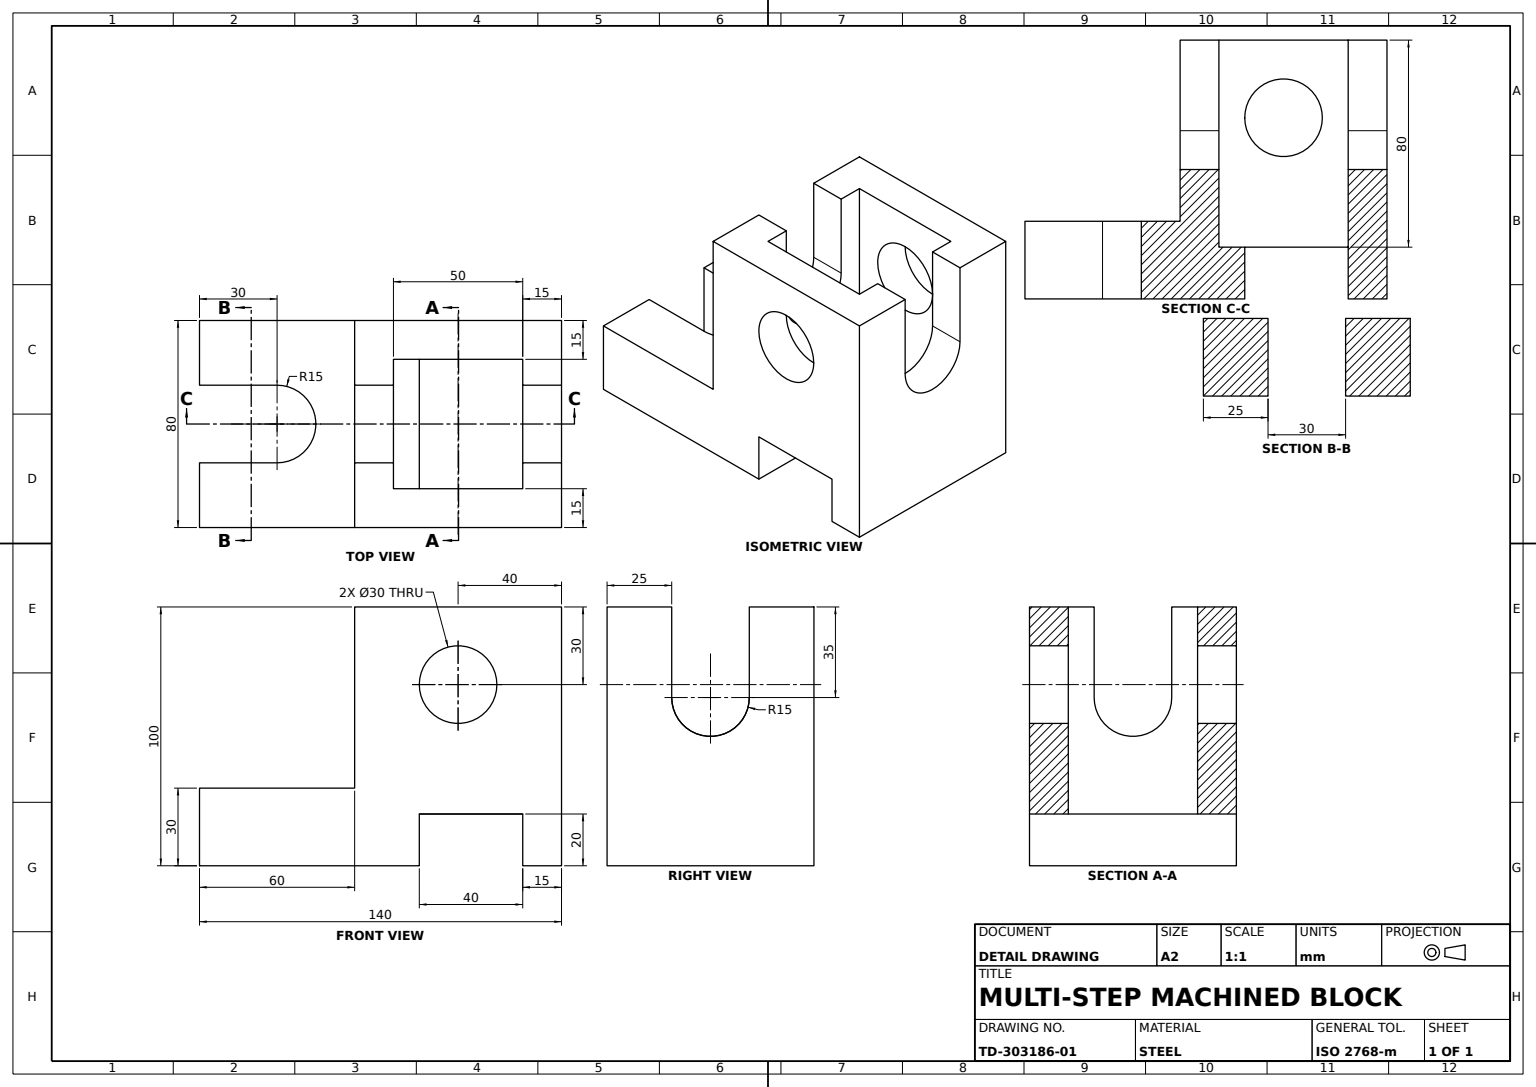
from build123d import *

# Parameters (mm, degrees)
BASE_BLOCK_SKETCH_W             = 140
BASE_BLOCK_SKETCH_H             = 30
BASE_BLOCK_DEPTH                = 80
BASE_NOTCH_SKETCH_W             = 40
BASE_NOTCH_SKETCH_H             = 20
BASE_NOTCH_DEPTH                = 80
UPRIGHT_SKETCH_W                = 80
UPRIGHT_SKETCH_H                = 70
UPRIGHT_DEPTH                   = 80
UPRIGHT_PROFILE_CUT_DEPTH       = 80
CROSS_HOLE_SKETCH_R             = 15
CROSS_HOLE_DEPTH                = 80
UPRIGHT_U_SLOT_DEPTH            = 80
BASE_UNDERSIDE_NOTCH_DEPTH      = 10
BASE_UNDERSIDE_NOTCH_DEPTH_BACK = 80


with BuildPart() as part:
    # Base Block Sketch → Base Block (new body)
    with BuildSketch(Plane.XY):
        with Locations((70, 15)):
            Rectangle(BASE_BLOCK_SKETCH_W, BASE_BLOCK_SKETCH_H)
    extrude(amount=-BASE_BLOCK_DEPTH)

    # Base Notch Sketch → Base Notch (cut)
    with BuildSketch(Plane.XY):
        with Locations((105, 10)):
            Rectangle(BASE_NOTCH_SKETCH_W, BASE_NOTCH_SKETCH_H)
    extrude(amount=-BASE_NOTCH_DEPTH, mode=Mode.SUBTRACT)

    # Upright Sketch → Upright (add)
    with BuildSketch(Plane.XY):
        with Locations((100, 65)):
            Rectangle(UPRIGHT_SKETCH_W, UPRIGHT_SKETCH_H)
    extrude(amount=-UPRIGHT_DEPTH)

    # Upright Profile Cut Sketch → Upright Profile Cut (cut)
    with BuildSketch(Plane(origin=(0, 100, 0), x_dir=(1, 0, 0), z_dir=(0, 1, 0))):
        Polygon((75, 15), (75, 40), (75, 65), (125, 65), (125, 15), align=None)
    extrude(amount=-UPRIGHT_PROFILE_CUT_DEPTH, mode=Mode.SUBTRACT)

    # Cross Hole Sketch → Cross Hole (cut)
    with BuildSketch(Plane.XY):
        with Locations((100, 70)):
            Circle(CROSS_HOLE_SKETCH_R)
    extrude(amount=-CROSS_HOLE_DEPTH, mode=Mode.SUBTRACT)

    # Upright U-Slot Sketch → Upright U-Slot (cut)
    with BuildSketch(Plane.ZY.offset(-60)):
        with BuildLine():
            Line((-25, 100), (-55, 100))
            Line((-55, 100), (-55, 65))
            ThreePointArc((-55, 65), (-40, 50), (-25, 65))
            Line((-25, 65), (-25, 100))
        make_face()
    extrude(amount=-UPRIGHT_U_SLOT_DEPTH, mode=Mode.SUBTRACT)

    # Base Underside Notch Sketch → Base Underside Notch (cut, two sides: drawn at the far end of the back side and taken through both)
    with BuildSketch(Plane(origin=(0, 30, 0), x_dir=(1, 0, 0), z_dir=(0, 1, 0)).offset(-BASE_UNDERSIDE_NOTCH_DEPTH_BACK)):
        with BuildLine():
            Line((30, 55), (0, 55))
            Line((0, 55), (0, 25))
            Line((0, 25), (30, 25))
            ThreePointArc((30, 25), (45, 40), (30, 55))
        make_face()
    extrude(amount=BASE_UNDERSIDE_NOTCH_DEPTH + BASE_UNDERSIDE_NOTCH_DEPTH_BACK, mode=Mode.SUBTRACT)


solid = part.part
